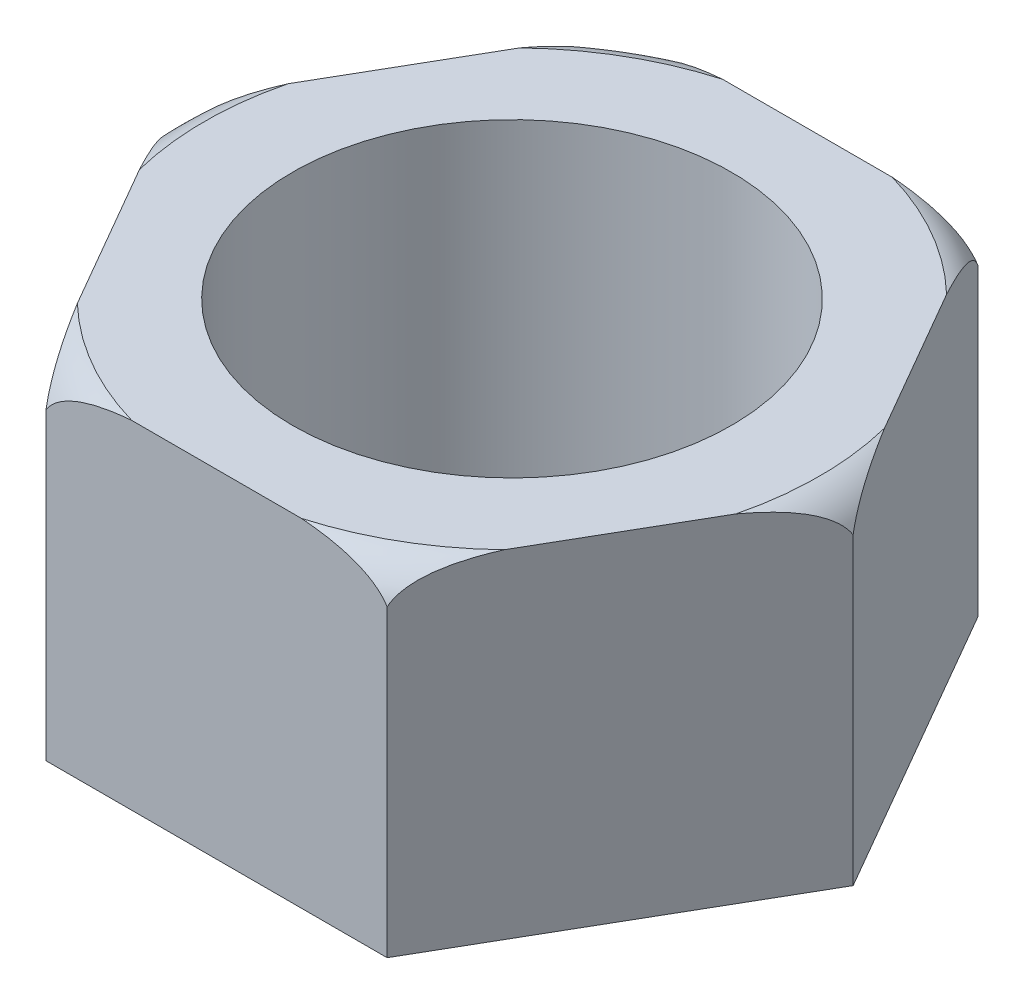
from build123d import *

# Parameters (mm, degrees)
HEX_PROFILE_SKETCH_R = 13
HEX_NUT_BODY_DEPTH   = 10


with BuildPart() as part:
    # Hex Profile Sketch → Hex Nut Body (new, symmetric)
    with BuildSketch(Plane(origin=(0, 0, 0), x_dir=(1, 0, 0), z_dir=(0, 1, 0))):
        Polygon((20.207259422, 0), (10.103629711, 17.5), (-10.103629711, 17.5), (-20.207259422, 0), (-10.103629711, -17.5), (10.103629711, -17.5), align=None)
        with Locations(Location((0, 0, 0), (0, 0, 270))):
            Circle(HEX_PROFILE_SKETCH_R, mode=Mode.SUBTRACT)
    extrude(amount=HEX_NUT_BODY_DEPTH, both=True)

    # Corner Chamfer Profile → Corner Chamfer Cut (revolve, cut)
    with BuildSketch(Plane.XY):
        with BuildLine():
            Line((18.207259422, 10), (20.207259422, 10))
            Line((20.207259422, 10), (20.207259422, 8))
            ThreePointArc((20.207259422, 8), (19.457751072, 9.25049165), (18.207259422, 10))
        make_face()
    revolve(axis=Axis((0, 0, 0), (0, 1, 0)), mode=Mode.SUBTRACT)


solid = part.part
